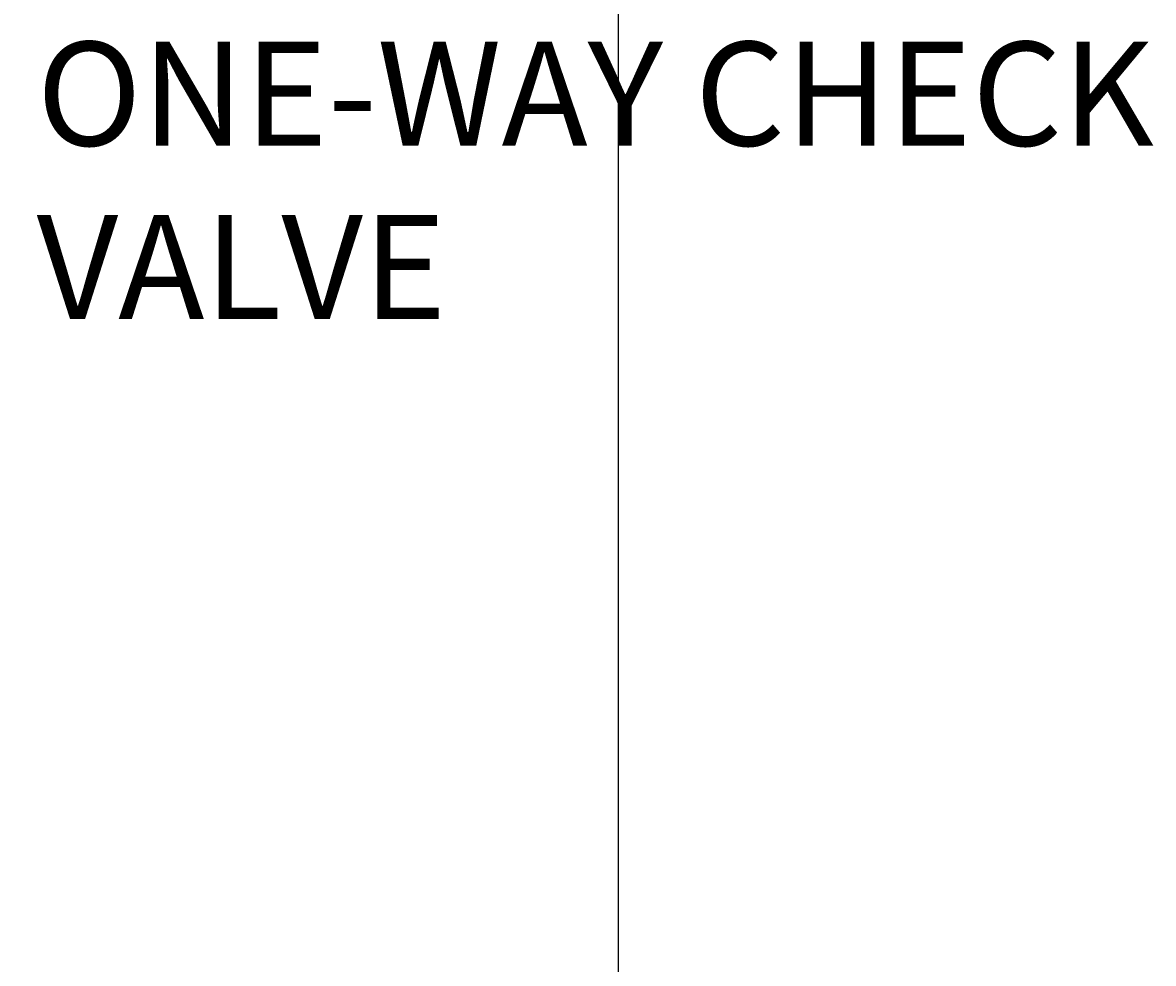
# Model space of a CAD drawing. Units: millimetres. Extents: x -11 to 280, y -4 to 208.
# Tile 53 of 55: x 237 to 280, y 106 to 142. Entities that reach past the tile are written whole.
import ezdxf

# ---------------------------------------------------------------- set-up
doc = ezdxf.new("R2010")
doc.units = ezdxf.units.MM
doc.layers.add('M-ANNO-TEXT', color=7, linetype='Continuous', lineweight=18)
doc.layers.add('M-DIMS', color=2, linetype='Continuous', lineweight=18)
doc.styles.get("Standard").update_dxf_attribs({"font": 'arial.ttf'})
doc.dimstyles.get("Standard").update_dxf_attribs({"dimtxt": 0.18, "dimasz": 0.18, "dimexe": 0.18, "dimexo": 0.0625, "dimgap": 0.09, "dimtad": 0, "dimtih": 1, "dimtoh": 1, "dimdec": 4, "dimzin": 0, "dimdsep": 46, "dimtxsty": 'Standard', "dimcen": 0.09, "dimadec": 0, "dimazin": 0, "dimtfac": 1, "dimtdec": 4, "dimtofl": 0, "dimtmove": 0, "dimatfit": 3, "dimfxl": 1, "dimtolj": 1, "dimtzin": 0, "dimarcsym": 0})

# ---------------------------------------------------------------- blocks, each defined once
blk = doc.blocks.new('*D5')
at = {"layer": 'Defpoints', "color": 0, "transparency": 16777216}
for p in [(24.759, 192.645), (-10.087, 11.435), (261.686, 11.435)]:
    blk.add_point(p, dxfattribs=at)
at = {"layer": 'M-DIMS', "color": 0, "lineweight": -2, "transparency": 16777216}
for p, q in [((24.696, 192.645), (-10.267, 192.645)), ((-10.087, 192.465), (-10.087, 102.222)), ((-10.087, 11.615), (-10.087, 101.858)), ((261.624, 11.435), (-10.267, 11.435))]:
    blk.add_line(p, q, dxfattribs=at)
at = {"layer": 'M-DIMS', "color": 0, "transparency": 16777216}
for points in [[(-10.117, 192.465), (-10.057, 192.465), (-10.087, 192.645)], [(-10.117, 11.615), (-10.057, 11.615), (-10.087, 11.435)]]:
    blk.add_solid(points, dxfattribs=at)
at = {"layer": 'M-DIMS', "color": 0, "transparency": 16777216, "insert": (-10.087, 102.04), "char_height": 0.18, "attachment_point": 5}
blk.add_mtext('\\A1;181.2', dxfattribs=at)
blk = doc.blocks.new('*D22')
at = {"layer": 'Defpoints', "color": 0, "transparency": 16777216}
for p in [(259.871, 207.495), (231.68, 34.723), (259.871, 34.723)]:
    blk.add_point(p, dxfattribs=at)
at = {"layer": 'M-DIMS', "color": 0, "lineweight": -2, "transparency": 16777216}
for p, q in [((231.68, 34.785), (231.68, 207.675)), ((259.871, 34.785), (259.871, 207.675)), ((231.86, 207.495), (245.38, 207.495)), ((259.691, 207.495), (246.171, 207.495))]:
    blk.add_line(p, q, dxfattribs=at)
at = {"layer": 'M-DIMS', "color": 0, "transparency": 16777216}
for points in [[(231.86, 207.525), (231.86, 207.465), (231.68, 207.495)], [(259.691, 207.525), (259.691, 207.465), (259.871, 207.495)]]:
    blk.add_solid(points, dxfattribs=at)
at = {"layer": 'M-DIMS', "color": 0, "transparency": 16777216, "insert": (245.776, 207.495), "char_height": 0.18, "attachment_point": 5}
blk.add_mtext('\\A1;28.19', dxfattribs=at)

msp = doc.modelspace()

# ---------------------------------------------------------------- texts
at = {"layer": 'M-ANNO-TEXT', "insert": (237.4756, 141.3233), "char_height": 4, "attachment_point": 1}
msp.add_mtext_dynamic_manual_height_columns('ONE-WAY CHECK\\PVALVE', width=63.617875, gutter_width=12.5, heights=[17.4015], dxfattribs=at)

# ---------------------------------------------------------------- dimensions: what is measured, and where the dimension line sits
at = {"layer": 'M-DIMS'}
dim = msp.add_linear_dim(base=(259.871, 207.495), p1=(231.6803, 34.7226), p2=(259.871, 34.7226), dimstyle='Standard', override={"dimdec": 2, "dimlfac": 1, "dimrnd": 0, "dimzin": 0, "dimdsep": 46, "dimlunit": 2}, dxfattribs=at)
dim.commit()
dim.dimension.update_dxf_attribs({"geometry": '*D22', "text_midpoint": (245.7757, 207.495)})
dim = msp.add_linear_dim(base=(-10.0865, 11.4346), p1=(24.7588, 192.645), p2=(261.6863, 11.4346), angle=90, dimstyle='Standard', override={"dimdec": 1, "dimlfac": 1, "dimrnd": 0, "dimzin": 0, "dimdsep": 46, "dimlunit": 2}, dxfattribs=at)
dim.commit()
dim.dimension.update_dxf_attribs({"geometry": '*D5', "text_midpoint": (-10.0865, 102.0398)})

doc.saveas('drawing.dxf')
